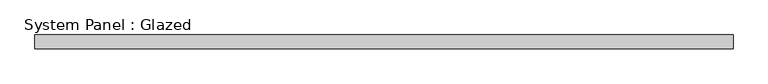
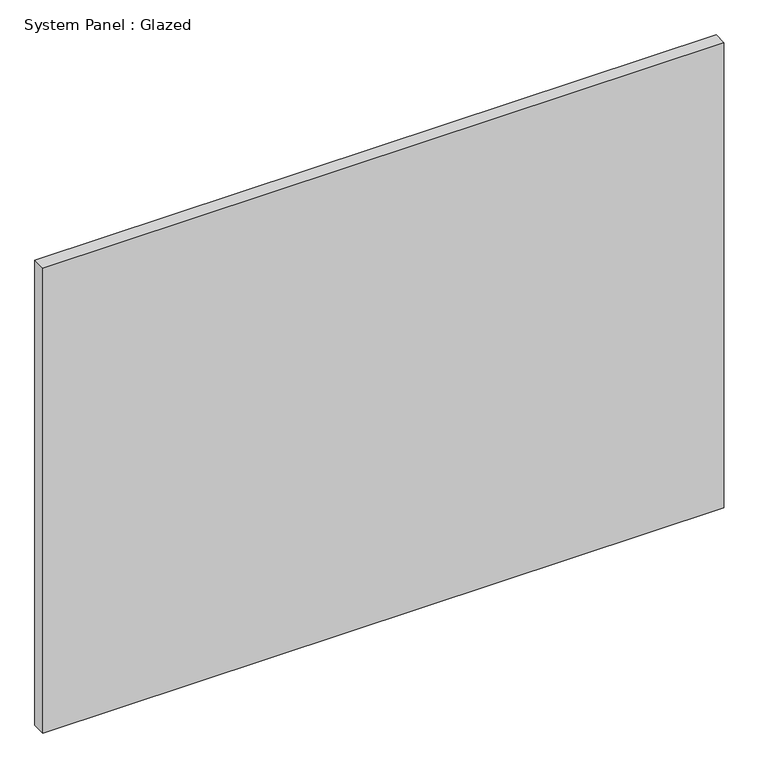
"""IFC4 building model written with IfcOpenShell, lengths in millimetres: plate geometry, System Panel : Glazed."""

from ifc_helpers import new_model, si_unit, origin, origin_with_axes, place, context, project, spatial, polyline, outline, extrude, source, transform, mapped, element, save


def system_panel_glazed_a8af599a(model_context):
    return source(origin(), model_context, "Body", "SweptSolid", [
        extrude(outline(polyline([(638.1750001, 19.05), (-638.1750001, 19.05), (-638.1750001, 44.45), (638.1750001, 44.45), (638.1750001, 19.05)])), origin_with_axes(), (0.0, 0.0, 1.0), 920.75),
    ])


if __name__ == "__main__":
    model = new_model("IFC4")
    model_context = context("Model", 3, world=origin())
    ifc_project = project(units=[si_unit("LENGTHUNIT", "METRE", prefix="MILLI")], contexts=[model_context])
    site = spatial("IfcSite", under=ifc_project)
    building = spatial("IfcBuilding", under=site)
    placement = place(None, origin())
    system_panel_glazed_shape = system_panel_glazed_a8af599a(model_context)
    element("IfcPlate", 1, ObjectType="System Panel : Glazed", at=placement, inside=building, context=model_context, shape_type="MappedRepresentation", body=[
        mapped(system_panel_glazed_shape, transform((0.0, 0.0, 0.0), x_axis=(1.0, 0.0, 0.0), y_axis=(0.0, 1.0, 0.0), z_axis=(0.0, 0.0, 1.0))),
    ])
    save(model, "model.ifc")

# Revit data of these elements
# Type "System Panel : Glazed"
#   Construction Type Id = "GSP4R"
#   Analytic Construction = "1/8 in Pilkington single glazing"
#   Visual Light Transmittance = 0.9
#   Solar Heat Gain Coefficient = 0.86
#   Heat Transfer Coefficient (U) = 1.18115 BTU/(h·ft²·°F)
#   Define Thermal Properties by = 1
# Element 1 (IfcPlate, "System Panel : Glazed")
#   Materials on its faces: "glass panel 223"
# Materials
#   "glass panel 223": class "Generic", colour RGB 120 120 120, transparency 0, Cost = 0
